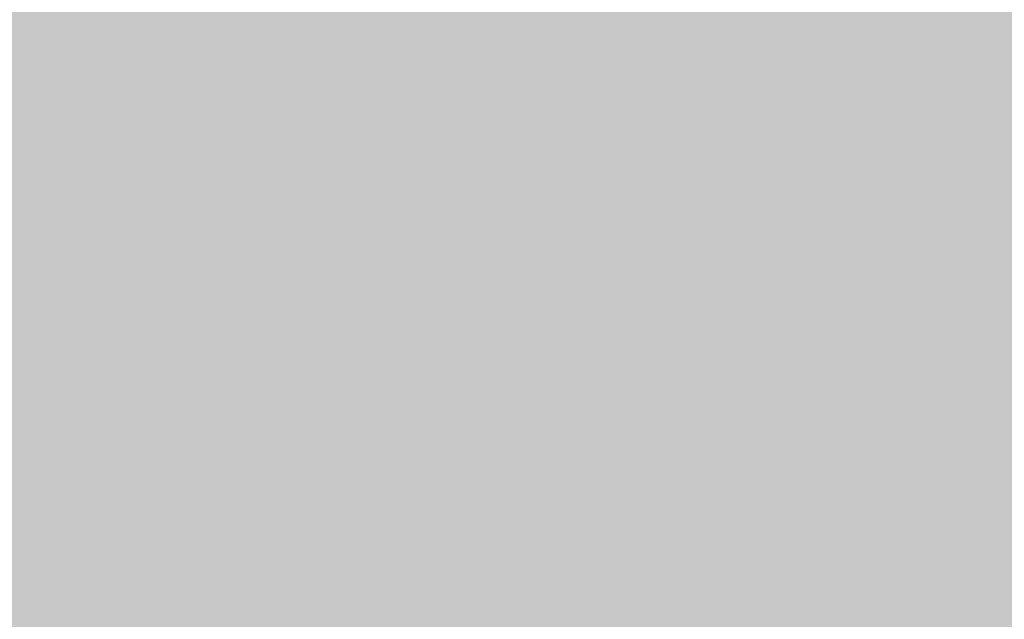
# Model space of a CAD drawing. Units: feet. Extents: x 3168 to 4724, y 827 to 1477.
# Tile 58 of 256: x 3273.143144 to 3273.145496, y 1099.01485 to 1099.016281. Entities that reach past the tile are written whole.
import ezdxf

# ---------------------------------------------------------------- set-up
doc = ezdxf.new("R2010")
doc.units = ezdxf.units.FT
doc.layers.add('A-ELEV', color=7, linetype='Continuous', lineweight=35)
doc.layers.add('A-ELEV-PATT', color=8, linetype='Continuous', lineweight=13)

msp = doc.modelspace()

# ---------------------------------------------------------------- hatches: boundary and pattern name
at = {"layer": 'A-ELEV-PATT'}
h = msp.add_hatch(color=256, dxfattribs=at)
h.dxf.hatch_style = 1
edge = h.paths.add_edge_path()
edge.add_ellipse((3552.9057615, 979.2201412), major_axis=(36.7449243, 0), ratio=0.4848484848, start_angle=0, end_angle=360)
edge = h.paths.add_edge_path()
edge.add_ellipse((3559.8916366, 929.2522824), major_axis=(36.7449243, 0), ratio=0.4848484848, start_angle=0, end_angle=360)
edge = h.paths.add_edge_path()
edge.add_line((3299.3168105, 1198.606081), (3479.9167135, 1198.606081))
edge.add_line((3479.9167135, 1198.606081), (3479.9167135, 1209.8685704))
edge.add_spline(control_points=[(3479.9167135, 1209.8685704), (3464.3011571, 1209.8685704), (3448.6856007, 1209.8685704), (3410.949139, 1209.8685704), (3388.8282339, 1209.8685704), (3355.6468761, 1209.8685704), (3344.5864235, 1209.8685704), (3327.9957446, 1209.8685704), (3322.4655183, 1209.8685704), (3314.1701788, 1209.8685704), (3311.4050657, 1209.8685704), (3307.257396, 1209.8685704), (3305.8748394, 1209.8685704), (3303.8010045, 1209.8685704), (3303.1097262, 1209.8685704), (3302.0728088, 1209.8685704), (3301.7271697, 1209.8685704), (3301.2087109, 1209.8685704), (3301.0358914, 1209.8685704), (3300.776662, 1209.8685704), (3300.6902522, 1209.8685704), (3300.5606376, 1209.8685704), (3300.5174327, 1209.8685704), (3300.4526253, 1209.8685704), (3300.4310229, 1209.8685704), (3300.3986192, 1209.8685704), (3300.387818, 1209.8685704), (3300.3662155, 1209.8685704), (3300.3456757, 1209.8685704), (3300.3455476, 1209.8685704), (3300.345505, 1209.8685704), (3300.3433041, 1209.8685704), (3300.341146, 1209.8685707), (3300.337909, 1209.8685714), (3300.33683, 1209.8685718), (3300.3339422, 1209.8685728), (3300.3321334, 1209.8685736), (3300.3255154, 1209.8685773), (3300.3207065, 1209.8685812), (3300.3109248, 1209.8685917), (3300.305952, 1209.8685984), (3300.2905113, 1209.8686233), (3300.2800452, 1209.8686461), (3300.2324255, 1209.868777), (3300.1952979, 1209.868954), (3299.9510684, 1209.8706077), (3299.7448244, 1209.8743259), (3299.4368271, 1209.8832566), (3299.3343894, 1209.8867924), (3299.181079, 1209.8929197), (3299.1300333, 1209.8950994), (3298.6522171, 1209.9168011), (3298.2294605, 1209.9457176), (3297.6016312, 1210.0023671), (3297.3934043, 1210.0234637), (3297.082652, 1210.058309), (3296.9793324, 1210.0704575), (3296.2929541, 1210.1548606), (3295.7181475, 1210.2433556), (3294.8687167, 1210.3988504), (3294.5876997, 1210.4544779), (3294.1693407, 1210.5433488), (3294.0304153, 1210.5738777), (3291.7071487, 1211.1012), (3289.6535901, 1211.8134353), (3285.7762586, 1213.5639876), (3283.9514101, 1214.6034778), (3280.512159, 1216.9800798), (3278.8972407, 1218.3175918), (3276.3799143, 1220.829489), (3275.4160415, 1221.9177379), (3274.0393421, 1223.7076996), (3273.5810428, 1224.3495346), (3273.1432283, 1225.0163162)], knot_values=[39.119033, 39.119033, 39.119033, 39.119033, 39.286353, 39.286353, 39.523379, 39.523379, 39.641892, 39.641892, 39.701148, 39.701148, 39.730777, 39.730777, 39.745591, 39.745591, 39.752998, 39.752998, 39.756701, 39.756701, 39.758553, 39.758553, 39.759479, 39.759479, 39.759942, 39.759942, 39.760173, 39.760173, 39.760289, 39.760289, 39.760405, 39.760405, 39.760463, 39.760463, 39.763389, 39.763389, 39.764851, 39.764851, 39.767304, 39.767304, 39.773825, 39.773825, 39.78057, 39.78057, 39.79477, 39.79477, 39.845194, 39.845194, 40.126715, 40.126715, 40.267476, 40.267476, 40.337856, 40.337856, 40.927023, 40.927023, 41.221606, 41.221606, 41.368898, 41.368898, 42.202622, 42.202622, 42.619485, 42.619485, 42.827916, 42.827916, 46.118323, 46.118323, 49.408731, 49.408731, 52.699139, 52.699139, 54.927489, 54.927489, 56.104228, 56.104228, 56.104228, 56.104228], weights=[1, 1, 1, 1, 1, 1, 1, 1, 1, 1, 1, 1, 1, 1, 1, 1, 1, 1, 1, 1, 1, 1, 1, 1, 1, 1, 1, 1, 1, 1, 1, 1, 1, 1, 1, 1, 1, 1, 1, 1, 1, 1, 1, 1, 1, 1, 1, 1, 1, 1, 1, 1, 1, 1, 1, 1, 1, 1, 1, 1, 1, 1, 1, 1, 1, 1, 1, 1, 1, 1, 1, 1, 1, 1], degree=3, periodic=0)
edge.add_line((3273.1432283, 1225.0163162), (3273.1432283, 1099.0163162))
edge.add_line((3273.1432283, 1099.0163162), (3299.3168105, 1099.0163162))
edge.add_line((3299.3168105, 1099.0163162), (3299.3168105, 1198.606081))
edge = h.paths.add_edge_path()
edge.add_line((3304.7584434, 1324.15806), (3479.9167135, 1324.15806))
edge.add_line((3479.9167135, 1324.15806), (3479.9167135, 1335.7146184))
edge.add_line((3479.9167135, 1335.7146184), (3269.1616284, 1335.7146184))
edge.add_spline(control_points=[(3269.1616284, 1335.7146184), (3264.0242315, 1335.7146184), (3258.364118, 1328.9581888), (3259.2643109, 1323.9002743)], knot_values=[0, 0, 0, 0, 15.412191, 15.412191, 15.412191, 15.412191], degree=3, periodic=0)
edge.add_line((3259.2643109, 1323.9002743), (3265.5168487, 1288.7691348))
edge.add_line((3265.5168487, 1288.7691348), (3275.2651026, 1261.5456259))
edge.add_line((3275.2651026, 1261.5456259), (3304.7584434, 1261.5456259))
edge.add_line((3304.7584434, 1261.5456259), (3304.7584434, 1324.15806))
h = msp.add_hatch(color=256, dxfattribs=at)
h.dxf.hatch_style = 1
h.paths.add_polyline_path([(3384.5252473, 1099.0163162), (3335.0291678, 1099.0163162), (3299.3168105, 1099.0163162), (3273.1432283, 1099.0163162), (3217.5653642, 1099.0163162), (3168.0692847, 827.1162598), (3335.0291678, 827.1162598)])

# ---------------------------------------------------------------- linework, layer by layer
at = {"layer": 'A-ELEV'}
msp.add_open_spline([(3808.5202001, 1099.0163162), (3808.5202001, 1141.413235), (3808.5202001, 1183.8101539), (3808.5202001, 1226.6353244), (3808.5202001, 1227.0635761), (3808.5202001, 1227.4918279), (3811.491871, 1248.9946729), (3814.463542, 1270.497518), (3817.4652299, 1292.2175635), (3817.4952467, 1292.434764), (3817.5252636, 1292.6519644), (3817.5728014, 1310.1067483), (3817.6203393, 1327.5615322), (3817.6678771, 1345.0163162), (3817.6678771, 1345.4579619), (3817.6678771, 1345.8996077), (3817.6678771, 1346.4560466), (3817.6678771, 1346.5708398), (3817.6678771, 1346.7528874), (3817.6678771, 1346.8201418), (3817.6678771, 1346.9348705), (3817.6678771, 1346.9823447), (3817.6678771, 1347.0385872), (3817.6678771, 1347.0473556), (3817.6678771, 1347.0736607), (3817.667877, 1347.0593025), (3817.6678766, 1347.0615455), (3817.6678764, 1347.0626669), (3817.6678754, 1347.0660311), (3817.6678743, 1347.0682738), (3817.6678701, 1347.0750012), (3817.667866, 1347.0794856), (3817.6678493, 1347.0929368), (3817.6678325, 1347.1019019), (3817.6677657, 1347.1287896), (3817.6676988, 1347.1467049), (3817.6674317, 1347.2004211), (3817.6671649, 1347.2361922), (3817.6661003, 1347.3433849), (3817.6650383, 1347.4146859), (3817.6608124, 1347.6280949), (3817.6566084, 1347.7697085), (3817.6399698, 1348.1924868), (3817.6235091, 1348.4715855), (3817.5590944, 1349.3000666), (3817.4961208, 1349.8405878), (3817.2554319, 1351.4241561), (3817.0263177, 1352.4287852), (3816.3068713, 1354.8889138), (3815.7437452, 1356.2687272), (3814.4639586, 1358.8192105), (3813.7464132, 1359.9909676), (3812.1958378, 1362.1723433), (3811.3622453, 1363.1821237), (3809.5888357, 1365.0690087), (3808.6488164, 1365.9461052), (3806.6542623, 1367.5796162), (3805.5997024, 1368.336154), (3803.3528906, 1369.7223272), (3802.1605354, 1370.352386), (3799.6008131, 1371.4535864), (3798.2326878, 1371.9254812), (3795.2800838, 1372.6346239), (3793.6931479, 1372.8720685), (3791.8694413, 1372.9264797), (3791.7408615, 1372.9292203), (3791.3533713, 1372.9341014), (3791.0927074, 1372.9329013), (3790.3041163, 1372.9150676), (3789.7695426, 1372.8841946), (3789.20919, 1372.8302363), (3789.1906217, 1372.8284241), (3789.1348916, 1372.8229123), (3789.097705, 1372.8191375), (3789.0484446, 1372.8140077), (3789.0364001, 1372.8127432), (3789.0002562, 1372.808918), (3788.9761468, 1372.8063255), (3788.9494049, 1372.8034042), (3788.9467858, 1372.8031177), (3788.9425667, 1372.8026552), (3788.9409669, 1372.8024797), (3788.9385718, 1372.8022166), (3788.9377765, 1372.8021292), (3788.9353908, 1372.8018669), (3788.8675349, 1372.7944024), (3788.7568665, 1372.7822285), (3788.7015323, 1372.7761415), (3788.5355297, 1372.7578805), (3788.4248612, 1372.7457065), (3788.092856, 1372.7091846), (3787.8715192, 1372.6848366), (3787.2075086, 1372.6117927), (3786.764835, 1372.5630968), (3785.436814, 1372.417009), (3784.5514666, 1372.3196171), (3781.8954246, 1372.0274416), (3780.1247299, 1371.8326579), (3774.8126458, 1371.2483067), (3771.2712564, 1370.8587393), (3760.6470883, 1369.6900371), (3753.5643095, 1368.9109022), (3732.3159732, 1366.5734977), (3718.1504157, 1365.015228), (3694.0067577, 1362.3593262), (3684.0286573, 1361.2616941), (3674.0505568, 1360.1640619), (3664.6006617, 1360.1640619), (3655.1507666, 1360.1640619), (3626.8010812, 1360.1640619), (3607.9012909, 1360.1640619), (3551.2019201, 1360.1640619), (3513.4023395, 1360.1640619), (3467.7251817, 1360.1640619), (3459.8476045, 1360.1640619), (3436.2148727, 1360.1640619), (3420.4597182, 1360.1640619), (3373.1942547, 1360.1640619), (3341.6839457, 1360.1640619), (3302.8481616, 1360.1640619), (3295.5226865, 1360.1640619), (3286.0382916, 1360.1640619), (3283.8793719, 1360.1640619), (3277.4026128, 1360.1640619), (3273.0847733, 1360.1640619), (3267.7328511, 1360.1640619), (3266.6987684, 1360.1640619), (3263.5965201, 1360.1640619), (3261.5283546, 1360.1640619), (3259.2369429, 1360.1640619), (3259.0136967, 1360.1640619), (3258.3439582, 1360.1640619), (3257.8974658, 1360.1640619), (3257.4309979, 1360.1640619), (3257.4110224, 1360.1640619), (3257.3705735, 1360.1640619), (3257.3754695, 1360.1640619), (3257.3745975, 1360.1640619), (3257.3739371, 1360.1640618), (3257.3719559, 1360.1640616), (3257.3706351, 1360.1640613), (3257.366673, 1360.16406), (3257.3640318, 1360.1640586), (3257.3561088, 1360.1640529), (3257.3508277, 1360.1640469), (3257.3349869, 1360.1640226), (3257.3244299, 1360.163998), (3257.2927692, 1360.1638987), (3257.2716761, 1360.1637987), (3257.208439, 1360.1633975), (3257.1663373, 1360.1629953), (3257.0402058, 1360.1613882), (3256.9563493, 1360.1597827), (3256.705504, 1360.1533932), (3256.53924, 1360.1470361), (3256.0435702, 1360.1219156), (3255.717296, 1360.0971018), (3254.7524458, 1360.0004808), (3254.1279679, 1359.906513), (3252.1800666, 1359.5253322), (3250.9415739, 1359.1439911), (3248.6701751, 1358.2432905), (3247.6357388, 1357.7238339), (3245.7326321, 1356.6034712), (3244.8633884, 1356.0020595), (3243.2531076, 1354.7428655), (3242.511972, 1354.0847309), (3240.7510518, 1352.3447812), (3239.8009609, 1351.229574), (3238.0877694, 1348.8724402), (3237.3246853, 1347.6303552), (3235.9825098, 1344.9716321), (3235.4022051, 1343.554907), (3234.5910812, 1340.8154577), (3234.3108819, 1339.5435498), (3233.9764902, 1336.8025605), (3233.9221126, 1335.3308771), (3234.1489156, 1332.5912693), (3234.3495287, 1331.3672011), (3234.7198926, 1329.9993668), (3234.7524228, 1329.8833616), (3234.853619, 1329.5347966), (3234.9258923, 1329.301685), (3235.0248359, 1329.0025524), (3235.0469235, 1328.936928), (3235.0776388, 1328.8472393), (3235.0859239, 1328.8231979), (3235.1109389, 1328.7510642), (3235.1278282, 1328.7029624), (3235.1479919, 1328.6462418), (3235.1510592, 1328.6376324), (3235.1560959, 1328.6235265), (3235.1580611, 1328.6180301), (3235.1602094, 1328.6120302), (3235.1656119, 1328.596943), (3235.1800989, 1328.556486), (3235.190263, 1328.5281009), (3235.2207556, 1328.4429457), (3235.241084, 1328.3861755), (3235.3020692, 1328.215865), (3235.3427259, 1328.1023247), (3235.4646962, 1327.7617038), (3235.5460097, 1327.5346232), (3235.7899503, 1326.8533813), (3235.9525774, 1326.39922), (3236.4404586, 1325.0367362), (3236.7657127, 1324.1284137), (3237.7414751, 1321.4034462), (3238.3919833, 1319.5868011), (3240.3435081, 1314.136866), (3241.6445245, 1310.503576), (3245.547574, 1299.6037058), (3248.149607, 1292.3371257), (3255.955706, 1270.5373853), (3261.1597719, 1256.004225), (3267.3876177, 1238.6120011), (3268.4113975, 1235.7529374), (3269.5103781, 1232.6838639), (3269.5855789, 1232.473854), (3269.7066118, 1232.1358507), (3269.752444, 1232.0078573), (3269.8273289, 1231.7987296), (3269.8563817, 1231.7175953), (3269.9063247, 1231.5781217), (3269.927215, 1231.5197823), (3269.9724682, 1231.3934057), (3269.9968311, 1231.3253685), (3270.0265026, 1231.2425062), (3270.0318112, 1231.2276812), (3270.0402823, 1231.2040243), (3270.0392242, 1231.2069792), (3270.0393595, 1231.2066014), (3270.0394271, 1231.2064125), (3270.0396301, 1231.2058458), (3270.0397654, 1231.205468), (3270.0401713, 1231.2043346), (3270.040442, 1231.2035791), (3270.041254, 1231.2013125), (3270.0417955, 1231.1998016), (3270.0434203, 1231.195269), (3270.044504, 1231.1922477), (3270.0477563, 1231.1831849), (3270.0499263, 1231.1771446), (3270.0564418, 1231.1590283), (3270.0607927, 1231.146957), (3270.0738674, 1231.1107614), (3270.0826128, 1231.0866558), (3270.1089357, 1231.0144129), (3270.1265997, 1230.9663498), (3270.1799341, 1230.8224568), (3270.2159467, 1230.7269233), (3270.3253234, 1230.4415078), (3270.4000257, 1230.2528107), (3270.6292491, 1229.6914436), (3270.7888829, 1229.3235005), (3271.2864875, 1228.2383194), (3271.6430996, 1227.5397546), (3272.7758592, 1225.515277), (3273.6141694, 1224.2605021), (3275.4160415, 1221.9177379), (3276.3799143, 1220.829489), (3278.8972407, 1218.3175918), (3280.512159, 1216.9800798), (3283.9514101, 1214.6034778), (3285.7762586, 1213.5639876), (3289.6535901, 1211.8134353), (3291.7071487, 1211.1012), (3294.0304153, 1210.5738777), (3294.1693407, 1210.5433488), (3294.5876997, 1210.4544779), (3294.8687167, 1210.3988504), (3295.7181475, 1210.2433556), (3296.2929541, 1210.1548606), (3296.9793324, 1210.0704575), (3297.082652, 1210.058309), (3297.3934043, 1210.0234637), (3297.6016312, 1210.0023671), (3298.2294605, 1209.9457176), (3298.6522171, 1209.9168011), (3299.1300333, 1209.8950994), (3299.181079, 1209.8929197), (3299.3343894, 1209.8867924), (3299.4368271, 1209.8832566), (3299.7448244, 1209.8743259), (3299.9510684, 1209.8706077), (3300.1952979, 1209.868954), (3300.2324255, 1209.868777), (3300.2800452, 1209.8686461), (3300.2905113, 1209.8686233), (3300.305952, 1209.8685984), (3300.3109248, 1209.8685917), (3300.3207065, 1209.8685812), (3300.3255154, 1209.8685773), (3300.3321334, 1209.8685736), (3300.3339422, 1209.8685728), (3300.33683, 1209.8685718), (3300.337909, 1209.8685714), (3300.341146, 1209.8685707), (3300.3433041, 1209.8685704), (3300.345505, 1209.8685704), (3300.3455476, 1209.8685704), (3300.3456757, 1209.8685704), (3300.3662155, 1209.8685704), (3300.387818, 1209.8685704), (3300.3986192, 1209.8685704), (3300.4310229, 1209.8685704), (3300.4526253, 1209.8685704), (3300.5174327, 1209.8685704), (3300.5606376, 1209.8685704), (3300.6902522, 1209.8685704), (3300.776662, 1209.8685704), (3301.0358914, 1209.8685704), (3301.2087109, 1209.8685704), (3301.7271697, 1209.8685704), (3302.0728088, 1209.8685704), (3303.1097262, 1209.8685704), (3303.8010045, 1209.8685704), (3305.8748394, 1209.8685704), (3307.257396, 1209.8685704), (3311.4050657, 1209.8685704), (3314.1701788, 1209.8685704), (3322.4655183, 1209.8685704), (3327.9957446, 1209.8685704), (3344.5864235, 1209.8685704), (3355.6468761, 1209.8685704), (3388.8282339, 1209.8685704), (3410.949139, 1209.8685704), (3477.3118546, 1209.8685704), (3521.553665, 1209.8685704), (3566.8361836, 1209.8685704), (3567.8768919, 1209.8685704), (3570.9990167, 1209.8685704), (3573.0804332, 1209.8685704), (3575.7813964, 1209.8685704), (3576.4009432, 1209.8685704), (3577.2958211, 1209.8685704), (3577.5711523, 1209.8685704), (3578.3971458, 1209.8685704), (3578.9478081, 1209.8685704), (3579.7564907, 1209.8685704), (3580.0145108, 1209.8685704), (3580.3427367, 1209.8685704), (3580.3268649, 1209.8685704), (3580.3271702, 1209.8685704), (3580.3273229, 1209.8685704), (3580.3277809, 1209.8685704), (3580.3280863, 1209.8685704), (3580.3290024, 1209.8685703), (3580.3296132, 1209.8685702), (3580.3314455, 1209.8685699), (3580.332667, 1209.8685697), (3580.336332, 1209.8685685), (3580.3387755, 1209.8685674), (3580.3461066, 1209.8685629), (3580.350995, 1209.8685584), (3580.3656627, 1209.8685402), (3580.3754446, 1209.868522), (3580.4048012, 1209.8684493), (3580.4243863, 1209.8683764), (3580.4831833, 1209.8680848), (3580.5224371, 1209.8677929), (3580.6403612, 1209.8666242), (3580.7191947, 1209.8654543), (3580.9563152, 1209.8607663), (3581.1152222, 1209.85607), (3581.5941635, 1209.8372298), (3581.9164188, 1209.8183314), (3582.8899466, 1209.7424284), (3583.547986, 1209.6661692), (3585.5318268, 1209.3606172), (3586.8672159, 1209.0538859), (3589.4715454, 1208.2524717), (3590.7402412, 1207.7578521), (3591.9954511, 1207.1588024), (3592.057809, 1207.1287398), (3592.2442418, 1207.0379536), (3592.3676757, 1206.9766317), (3592.73528, 1206.7903591), (3592.9767518, 1206.663101), (3593.2445387, 1206.5164414), (3593.2747313, 1206.4998248), (3593.3651153, 1206.4498388), (3593.4251129, 1206.4163333), (3593.6043138, 1206.3152851), (3593.7227254, 1206.2472105), (3593.8572122, 1206.1683978), (3593.8743621, 1206.1583193), (3593.925741, 1206.1280407), (3593.9598989, 1206.1077976), (3594.0620855, 1206.0468991), (3594.1298272, 1206.0060745), (3594.2084359, 1205.9581709), (3594.2196829, 1205.9513043), (3594.253391, 1205.9306863), (3594.2758193, 1205.9169166), (3594.3429716, 1205.8755358), (3594.3875633, 1205.8478526), (3594.4336161, 1205.8190499), (3594.4352559, 1205.818024), (3594.4401746, 1205.8149461), (3594.4434527, 1205.8128936), (3594.4471229, 1205.8105944), (3594.4475159, 1205.8103482), (3594.4486949, 1205.8096095), (3594.4494808, 1205.8091171), (3594.4503663, 1205.8085621), (3594.4504658, 1205.8084998), (3594.4506003, 1205.8084155), (3594.4673993, 1205.7978872), (3594.4932689, 1205.7816741), (3594.5062037, 1205.7735675), (3594.5450081, 1205.7492479), (3594.5708778, 1205.7330348), (3594.6484866, 1205.6843956), (3594.7002258, 1205.6519694), (3594.8554436, 1205.5546909), (3594.958922, 1205.4898386), (3595.2693574, 1205.2952816), (3595.4763144, 1205.1655769), (3596.0971852, 1204.7764629), (3596.5110991, 1204.5170536), (3597.7528407, 1203.7388256), (3598.5806685, 1203.220007), (3601.0641518, 1201.663551), (3602.7198073, 1200.6259137), (3607.686774, 1197.5130018), (3610.998085, 1195.4377272), (3620.9320182, 1189.2119034), (3627.5546404, 1185.0613542), (3647.4225068, 1172.6097066), (3660.6677511, 1164.3086082), (3700.403484, 1139.405313), (3726.8939725, 1122.8031161), (3757.2057154, 1103.8060516), (3761.0269697, 1101.4111839), (3764.848224, 1099.0163162), (3745.3282713, 1099.0163162), (3725.8083186, 1099.0163162), (3706.288366, 1099.0163162), (3706.288366, 1108.4532371), (3706.288366, 1117.890158), (3706.288366, 1127.3270789), (3710.7507544, 1127.3270789), (3715.2131428, 1127.3270789), (3719.6755312, 1127.3270789)], degree=3, knots=[0, 0, 0, 0, 0.982037, 0.982037, 0.991957, 0.991957, 0.991957, 1.966522, 1.966522, 1.976367, 1.976367, 1.976367, 2.976367, 2.976367, 2.976367, 3.00169, 3.00169, 3.008272, 3.008272, 3.012129, 3.012129, 3.014851, 3.014851, 3.015353, 3.015353, 3.016359, 3.016359, 3.017365, 3.017365, 3.019376, 3.019376, 3.023398, 3.023398, 3.031442, 3.031442, 3.047531, 3.047531, 3.079708, 3.079708, 3.144063, 3.144063, 3.272772, 3.272772, 3.53019, 3.53019, 4.045026, 4.045026, 5.074698, 5.074698, 6.700878, 6.700878, 8.327058, 8.327058, 9.953238, 9.953238, 11.579418, 11.579418, 13.205598, 13.205598, 14.831778, 14.831778, 16.457958, 16.457958, 18.084138, 18.084138, 18.206872, 18.206872, 18.45234, 18.45234, 18.943275, 18.943275, 18.960093, 18.960093, 18.993729, 18.993729, 19.00461, 19.00461, 19.026374, 19.026374, 19.028737, 19.028737, 19.03018, 19.03018, 19.030897, 19.030897, 19.032332, 19.032332, 19.033766, 19.033766, 19.036636, 19.036636, 19.042374, 19.042374, 19.053851, 19.053851, 19.076805, 19.076805, 19.122714, 19.122714, 19.21453, 19.21453, 19.398163, 19.398163, 19.765429, 19.765429, 20.024128, 20.024128, 20.024128, 20.092031, 20.092031, 20.227836, 20.227836, 20.499446, 20.499446, 20.556051, 20.556051, 20.66926, 20.66926, 20.895678, 20.895678, 20.948316, 20.948316, 20.963829, 20.963829, 20.994855, 20.994855, 21.002285, 21.002285, 21.017146, 21.017146, 21.01875, 21.01875, 21.021959, 21.021959, 21.022102, 21.022102, 21.022249, 21.022249, 21.022708, 21.022708, 21.023627, 21.023627, 21.025464, 21.025464, 21.029138, 21.029138, 21.036486, 21.036486, 21.051183, 21.051183, 21.080575, 21.080575, 21.139361, 21.139361, 21.256932, 21.256932, 21.492073, 21.492073, 21.962356, 21.962356, 23.01002, 23.01002, 24.057684, 24.057684, 25.105348, 25.105348, 26.153011, 26.153011, 27.776787, 27.776787, 29.400562, 29.400562, 31.024337, 31.024337, 32.278801, 32.278801, 33.533265, 33.533265, 34.467568, 34.467568, 34.553971, 34.553971, 34.726776, 34.726776, 34.775309, 34.775309, 34.793079, 34.793079, 34.82862, 34.82862, 34.834979, 34.834979, 34.839039, 34.839039, 34.839411, 34.839411, 34.840285, 34.840285, 34.842034, 34.842034, 34.845531, 34.845531, 34.852525, 34.852525, 34.866512, 34.866512, 34.894488, 34.894488, 34.950439, 34.950439, 35.062342, 35.062342, 35.286147, 35.286147, 35.733758, 35.733758, 35.821815, 35.821815, 35.828283, 35.828283, 35.832225, 35.832225, 35.834724, 35.834724, 35.836521, 35.836521, 35.838617, 35.838617, 35.839073, 35.839073, 35.839345, 35.839345, 35.839617, 35.839617, 35.840161, 35.840161, 35.841249, 35.841249, 35.843425, 35.843425, 35.847778, 35.847778, 35.856482, 35.856482, 35.873891, 35.873891, 35.908709, 35.908709, 35.978345, 35.978345, 36.117617, 36.117617, 36.396161, 36.396161, 36.953248, 36.953248, 38.067423, 38.067423, 40.295772, 40.295772, 42.524122, 42.524122, 45.81453, 45.81453, 49.104937, 49.104937, 52.395345, 52.395345, 52.603776, 52.603776, 53.020639, 53.020639, 53.854363, 53.854363, 54.001655, 54.001655, 54.296238, 54.296238, 54.885405, 54.885405, 54.955785, 54.955785, 55.096546, 55.096546, 55.378067, 55.378067, 55.42849, 55.42849, 55.442691, 55.442691, 55.449436, 55.449436, 55.455957, 55.455957, 55.458409, 55.458409, 55.459872, 55.459872, 55.462798, 55.462798, 55.462856, 55.462856, 55.462972, 55.462972, 55.463088, 55.463088, 55.463319, 55.463319, 55.463782, 55.463782, 55.464708, 55.464708, 55.46656, 55.46656, 55.470263, 55.470263, 55.47767, 55.47767, 55.492484, 55.492484, 55.522112, 55.522112, 55.581369, 55.581369, 55.699882, 55.699882, 55.936907, 55.936907, 56.410959, 56.410959, 56.42211, 56.42211, 56.444413, 56.444413, 56.451051, 56.451051, 56.454001, 56.454001, 56.459901, 56.459901, 56.462666, 56.462666, 56.463418, 56.463418, 56.464171, 56.464171, 56.465675, 56.465675, 56.468684, 56.468684, 56.474702, 56.474702, 56.486738, 56.486738, 56.51081, 56.51081, 56.558955, 56.558955, 56.655243, 56.655243, 56.847821, 56.847821, 57.232975, 57.232975, 58.003284, 58.003284, 59.543901, 59.543901, 62.625137, 62.625137, 68.787607, 68.787607, 74.950078, 74.950078, 75.27336, 75.27336, 75.919923, 75.919923, 77.213051, 77.213051, 77.377769, 77.377769, 77.707206, 77.707206, 78.366079, 78.366079, 78.462532, 78.462532, 78.655436, 78.655436, 79.041245, 79.041245, 79.105735, 79.105735, 79.234714, 79.234714, 79.492672, 79.492672, 79.502197, 79.502197, 79.521249, 79.521249, 79.523534, 79.523534, 79.528103, 79.528103, 79.528682, 79.528682, 79.528885, 79.528885, 79.529089, 79.529089, 79.529495, 79.529495, 79.530308, 79.530308, 79.531935, 79.531935, 79.535187, 79.535187, 79.541693, 79.541693, 79.554704, 79.554704, 79.580725, 79.580725, 79.632769, 79.632769, 79.736856, 79.736856, 79.94503, 79.94503, 80.361377, 80.361377, 80.421435, 80.421435, 80.421435, 81.421435, 81.421435, 81.421435, 82.421435, 82.421435, 82.421435, 83.421435, 83.421435, 83.421435, 83.421435], dxfattribs=at)

doc.saveas('drawing.dxf')
